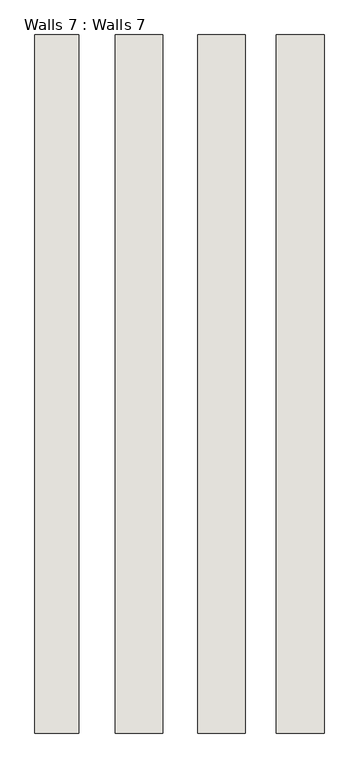
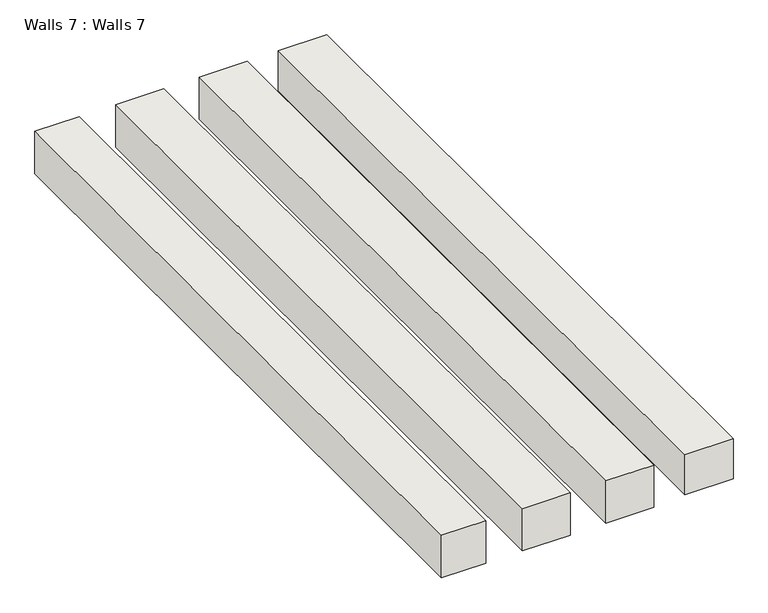
"""IFC4 building model written with IfcOpenShell, lengths in millimetres: wall geometry, Walls 7 : Walls 7."""

from ifc_helpers import new_model, si_unit, frame, origin, place, context, project, spatial, polyline, outline, extrude, source, transform, mapped, element, save


def walls_7_walls_7_6bd86e60(model_context):
    return source(origin(), model_context, "Body", "SweptSolid", [
        extrude(outline(polyline([(-8296.7748542, -2383.3885822), (-8522.6585036, -2383.3885822), (-8522.6585036, 1210.7114178), (-8296.7748542, 1210.7114178), (-8296.7748542, -2383.3885822)])), frame((0.0, 0.0, 11963.4), z_axis=(0.0, 0.0, 1.0), x_axis=(1.0, 0.0, 0.0)), (0.0, 0.0, 1.0), 228.6),
        extrude(outline(polyline([(-7864.9210028, -2383.3885822), (-8109.6381853, -2383.3885822), (-8109.6381853, 1210.7114178), (-7864.9210028, 1210.7114178), (-7864.9210028, -2383.3885822)])), frame((0.0, 0.0, 11963.4), z_axis=(0.0, 0.0, 1.0), x_axis=(1.0, 0.0, 0.0)), (0.0, 0.0, 1.0), 228.6),
        extrude(outline(polyline([(-7439.2364922, -2383.3885822), (-7683.9536746, -2383.3885822), (-7683.9536746, 1210.7114178), (-7439.2364922, 1210.7114178), (-7439.2364922, -2383.3885822)])), frame((0.0, 0.0, 11963.4), z_axis=(0.0, 0.0, 1.0), x_axis=(1.0, 0.0, 0.0)), (0.0, 0.0, 1.0), 228.6),
        extrude(outline(polyline([(-7034.1164507, -2383.3885822), (-7280.0192972, -2383.3885822), (-7280.0192972, 1210.7114178), (-7034.1164507, 1210.7114178), (-7034.1164507, -2383.3885822)])), frame((0.0, 0.0, 11976.1), z_axis=(0.0, 0.0, 1.0), x_axis=(1.0, 0.0, 0.0)), (0.0, 0.0, 1.0), 215.9),
    ])


if __name__ == "__main__":
    model = new_model("IFC4")
    model_context = context("Model", 3, world=origin())
    ifc_project = project(units=[si_unit("LENGTHUNIT", "METRE", prefix="MILLI")], contexts=[model_context])
    site = spatial("IfcSite", under=ifc_project)
    building = spatial("IfcBuilding", under=site)
    placement = place(None, origin())
    walls_7_walls_7_shape = walls_7_walls_7_6bd86e60(model_context)
    element("IfcWall", 1, ObjectType="Walls 7 : Walls 7", at=placement, inside=building, context=model_context, shape_type="MappedRepresentation", body=[
        mapped(walls_7_walls_7_shape, transform((0.0, 0.0, 0.0), x_axis=(1.0, 0.0, 0.0), y_axis=(0.0, 1.0, 0.0), z_axis=(0.0, 0.0, 1.0))),
    ])
    save(model, "model.ifc")

# Revit data of these elements
# Element 1 (IfcWall, "Walls 7 : Walls 7")
#   Materials on its faces: "Default Wall"
# Materials
#   "Default Wall": colour RGB 128 128 128, transparency 0
